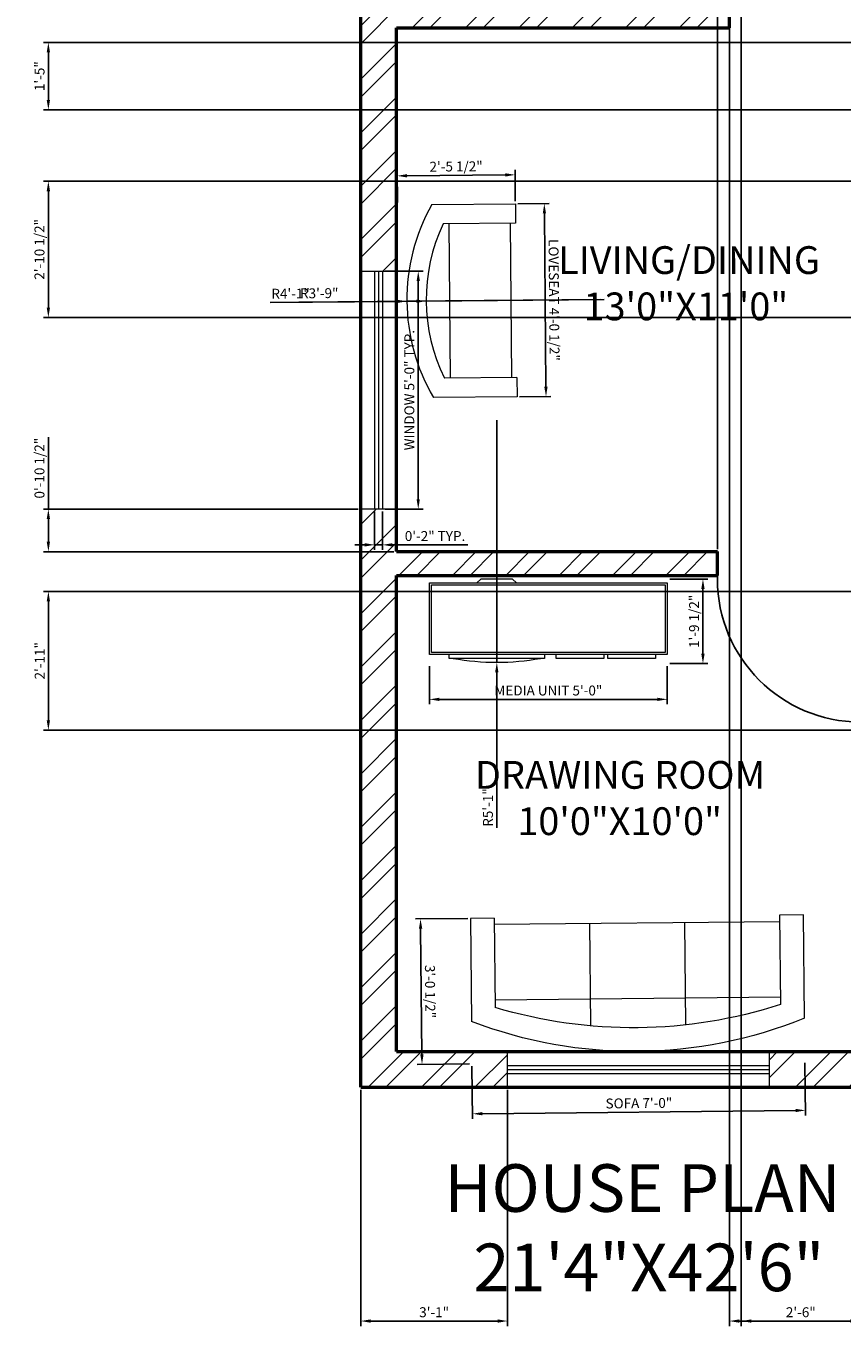
# Model space of a CAD drawing. Units: inches. Extents: x 1147 to 1568, y 1982 to 2559.
# Tile 1 of 4: x 1147 to 1353, y 1982 to 2309. Entities that reach past the tile are written whole.
import ezdxf

# ---------------------------------------------------------------- set-up
doc = ezdxf.new("R2010")
doc.units = ezdxf.units.IN
for name, color, linetype, lineweight in [('A-ANNO-DIMS', 2, 'Continuous', 18), ('A-DOOR', 4, 'Continuous', 25), ('A-WALL', 7, 'Continuous', 50), ('A-WALL-PATT', 252, 'Continuous', 13)]:
    doc.layers.add(name, color=color, linetype=linetype, lineweight=lineweight)
for name, color, linetype, lineweight, true_color in [('A-ANNO-TITL', 244, 'Continuous', 35, 0x991b1e), ('A-AREA-IDEN', 244, 'Continuous', 25, 0x991b1e), ('A-FURN', 244, 'Continuous', 18, 0x991b1e), ('A-GLAZ', 177, 'Continuous', 18, 0x293189)]:
    doc.layers.add(name, color=color, linetype=linetype, lineweight=lineweight, true_color=true_color)
doc.styles.get("Standard").update_dxf_attribs({"font": 'arial.ttf'})
doc.dimstyles.new('ISO-25', dxfattribs={"dimtxt": 2.5, "dimasz": 2.5, "dimexe": 1.25, "dimexo": 0.625, "dimtad": 1, "dimlunit": 3, "dimtxsty": 'Standard', "dimcen": 2.5, "dimadec": 0, "dimazin": 0, "dimtfac": 1, "dimtmove": 0, "dimatfit": 3, "dimfxl": 1, "dimarcsym": 0})

# ---------------------------------------------------------------- blocks, each defined once
blk = doc.blocks.new('*U3')
for p, q in [((-40, 0), (-40, 6)), ((0, 0), (0, 6))]:
    blk.add_line(p, q)
blk.add_lwpolyline([(0, 0), (0, -40), (-1.75, -40), (-1.75, 0)], close=True)
blk.add_arc((0, 0), 40, 180, 270)
blk = doc.blocks.new('Entertainment Center')
for p, q in [((-4, 0), (-5, -1)), ((4, 0), (-4, 0)), ((5, -1), (4, 0)), ((-17, -19), (-17, -1)), ((-17, -1), (43, -1)), ((-16.5, -18.5), (-16.5, -1.5)), ((-16.5, -1.5), (42.5, -1.5)), ((42.5, -1.5), (42.5, -18.5)), ((43, -1), (43, -19)), ((43, -19), (-17, -19)), ((42.5, -18.5), (-16.5, -18.5)), ((-12, -20), (-12, -19)), ((12, -19), (12, -20)), ((15, -20), (15, -19)), ((27, -19), (27, -20)), ((28, -20), (28, -19)), ((40, -19), (40, -20)), ((12, -20), (-12, -20)), ((27, -20), (15, -20)), ((40, -20), (28, -20))]:
    blk.add_line(p, q)
blk.add_arc((0, 40), 61, 259.6111, 280.3889)
blk = doc.blocks.new('Sofa - Roundback Loveseat 5 ft.')
for p, q in [((0, -32.44198), (0, -5.99998)), ((-24, -33.99998), (-24, -11.46958)), ((24.00004, -33.99998), (24.00004, -11.46958)), ((-23.9998, -13.38178), (23.99986, -13.38178)), ((-24, -32.44198), (24.00004, -32.44198))]:
    blk.add_line(p, q)
for points in [[(-24, -33.99998), (-30, -33.99998), (-30, -7.99998)], [(30.00004, -7.99998), (30.00004, -33.99998), (24.00004, -33.99998)]]:
    blk.add_lwpolyline(points)
for centre, radius, start, end in [((0, -60.24998), 60.24998, 60.13715, 119.8628), ((0, -61.38438), 55.38444, 64.32083, 115.6792)]:
    blk.add_arc(centre, radius, start, end)
blk = doc.blocks.new('Sofa - Roundback 7 ft.')
for p, q in [((-12.00002, -32.4421), (-12.00003, -6.5971)), ((11.99997, -32.4421), (11.99998, -6.5971)), ((-36.000027, -34), (-36.000027, -11.4696)), ((35.99998, -34), (35.99998, -11.4696)), ((-35.999844, -13.3819), (35.9998, -13.3819)), ((-36.000027, -32.4421), (35.99998, -32.4421))]:
    blk.add_line(p, q)
for points in [[(-36.000027, -34), (-42.000027, -34), (-42.000027, -8)], [(41.99998, -8), (41.99998, -34), (35.99998, -34)]]:
    blk.add_lwpolyline(points)
for centre, radius, start, end in [((0, -114.25), 114.25, 68.43141, 111.5686), ((-0.00001, -127.1968), 121.1968, 72.72033, 107.2797)]:
    blk.add_arc(centre, radius, start, end)
blk = doc.blocks.new('WIN-GLAZ-66IN')
for p, q in [((0, 2), (66, 2)), ((0, 1), (66, 1)), ((0, 0), (66, 0))]:
    blk.add_line(p, q)
blk = doc.blocks.new('WIN-GLAZ-60IN')
for p, q in [((0, 60), (0, 0)), ((1, 60), (1, 0)), ((2, 60), (2, 0))]:
    blk.add_line(p, q)
blk = doc.blocks.new('*D25')
at = {"layer": 'A-ANNO-DIMS', "color": 0, "lineweight": -2, "transparency": 16777216}
for p, q in [((1237.73, 2247.42), (1247.36, 2247.42)), ((1246.11, 2189.92), (1246.11, 2244.92)), ((1237.73, 2187.42), (1247.36, 2187.42))]:
    blk.add_line(p, q, dxfattribs=at)
at = {"layer": 'A-ANNO-DIMS', "color": 0, "transparency": 16777216}
for points in [[(1245.69, 2244.92), (1246.52, 2244.92), (1246.11, 2247.42)], [(1245.69, 2189.92), (1246.52, 2189.92), (1246.11, 2187.42)]]:
    blk.add_solid(points, dxfattribs=at)
at = {"layer": 'Defpoints', "color": 0, "transparency": 16777216}
for p in [(1237.11, 2247.42), (1246.11, 2247.42), (1237.11, 2187.42)]:
    blk.add_point(p, dxfattribs=at)
at = {"layer": 'A-ANNO-DIMS', "color": 0, "transparency": 16777216, "insert": (1244.19, 2217.42), "char_height": 2.5, "attachment_point": 5, "rotation": 90}
blk.add_mtext('WINDOW 5\'-0" TYP.', dxfattribs=at)
blk = doc.blocks.new('*D26')
at = {"layer": 'A-ANNO-DIMS', "color": 0, "lineweight": -2, "transparency": 16777216}
for p, q in [((1235.11, 2186.79), (1235.11, 2177.17)), ((1237.11, 2186.79), (1237.11, 2177.17)), ((1232.61, 2178.42), (1230.11, 2178.42)), ((1235.11, 2178.42), (1237.11, 2178.42)), ((1239.61, 2178.42), (1258.6, 2178.42))]:
    blk.add_line(p, q, dxfattribs=at)
at = {"layer": 'A-ANNO-DIMS', "color": 0, "transparency": 16777216}
for points in [[(1232.61, 2178.84), (1232.61, 2178), (1235.11, 2178.42)], [(1239.61, 2178.84), (1239.61, 2178), (1237.11, 2178.42)]]:
    blk.add_solid(points, dxfattribs=at)
at = {"layer": 'Defpoints', "color": 0, "transparency": 16777216}
for p in [(1235.11, 2187.42), (1237.11, 2187.42), (1237.11, 2178.42)]:
    blk.add_point(p, dxfattribs=at)
at = {"layer": 'A-ANNO-DIMS', "color": 0, "transparency": 16777216, "insert": (1250.35, 2180.32), "char_height": 2.5, "attachment_point": 5}
blk.add_mtext('0\'-2" TYP.', dxfattribs=at)
blk = doc.blocks.new('*D35')
at = {"layer": 'A-ANNO-DIMS', "color": 0, "lineweight": -2, "transparency": 16777216}
for p, q in [((1248.93, 2147.85), (1248.93, 2138.23)), ((1308.93, 2147.85), (1308.93, 2138.23)), ((1251.43, 2139.48), (1306.43, 2139.48))]:
    blk.add_line(p, q, dxfattribs=at)
at = {"layer": 'A-ANNO-DIMS', "color": 0, "transparency": 16777216}
for points in [[(1251.43, 2139.89), (1251.43, 2139.06), (1248.93, 2139.48)], [(1306.43, 2139.89), (1306.43, 2139.06), (1308.93, 2139.48)]]:
    blk.add_solid(points, dxfattribs=at)
at = {"layer": 'Defpoints', "color": 0, "transparency": 16777216}
for p in [(1248.93, 2148.48), (1308.93, 2148.48), (1308.93, 2139.48)]:
    blk.add_point(p, dxfattribs=at)
at = {"layer": 'A-ANNO-DIMS', "color": 0, "transparency": 16777216, "insert": (1278.93, 2141.38), "char_height": 2.5, "attachment_point": 5}
blk.add_mtext('MEDIA UNIT 5\'-0"', dxfattribs=at)
blk = doc.blocks.new('*D36')
at = {"layer": 'A-ANNO-DIMS', "color": 0, "lineweight": -2, "transparency": 16777216}
for p, q in [((1309.55, 2169.81), (1319.18, 2169.81)), ((1317.93, 2150.98), (1317.93, 2167.31)), ((1309.55, 2148.48), (1319.18, 2148.48))]:
    blk.add_line(p, q, dxfattribs=at)
at = {"layer": 'A-ANNO-DIMS', "color": 0, "transparency": 16777216}
for points in [[(1317.51, 2167.31), (1318.34, 2167.31), (1317.93, 2169.81)], [(1317.51, 2150.98), (1318.34, 2150.98), (1317.93, 2148.48)]]:
    blk.add_solid(points, dxfattribs=at)
at = {"layer": 'Defpoints', "color": 0, "transparency": 16777216}
for p in [(1308.93, 2169.81), (1317.93, 2169.81), (1308.93, 2148.48)]:
    blk.add_point(p, dxfattribs=at)
at = {"layer": 'A-ANNO-DIMS', "color": 0, "transparency": 16777216, "insert": (1316.01, 2159.14), "char_height": 2.5, "attachment_point": 5, "rotation": 90}
blk.add_mtext('1\'-9 1/2"', dxfattribs=at)
blk = doc.blocks.new('*D39')
at = {"layer": 'A-ANNO-DIMS', "color": 0, "lineweight": -2, "transparency": 16777216}
for p, q in [((1271.23, 2264.4), (1279.16, 2264.47)), ((1278.32, 2218.29), (1277.93, 2261.96)), ((1271.67, 2215.73), (1279.59, 2215.8))]:
    blk.add_line(p, q, dxfattribs=at)
at = {"layer": 'A-ANNO-DIMS', "color": 0, "transparency": 16777216}
for points in [[(1278.35, 2261.96), (1277.52, 2261.95), (1277.91, 2264.46)], [(1278.74, 2218.29), (1277.9, 2218.29), (1278.34, 2215.79)]]:
    blk.add_solid(points, dxfattribs=at)
at = {"layer": 'Defpoints', "color": 0, "transparency": 16777216}
for p in [(1270.61, 2264.39), (1277.91, 2264.46), (1271.04, 2215.72)]:
    blk.add_point(p, dxfattribs=at)
at = {"layer": 'A-ANNO-DIMS', "color": 0, "transparency": 16777216, "insert": (1280.04, 2240.14), "char_height": 2.5, "attachment_point": 5, "rotation": 270.5097}
blk.add_mtext('LOVESEAT 4\'-0 1/2"', dxfattribs=at)
blk = doc.blocks.new('*D40')
at = {"layer": 'A-ANNO-DIMS', "color": 0, "lineweight": -2, "transparency": 16777216}
for p, q in [((1240.86, 2264.75), (1240.79, 2272.68)), ((1268.05, 2271.67), (1243.3, 2271.45)), ((1270.6, 2265.02), (1270.53, 2272.94))]:
    blk.add_line(p, q, dxfattribs=at)
at = {"layer": 'A-ANNO-DIMS', "color": 0, "transparency": 16777216}
for points in [[(1243.3, 2271.87), (1243.31, 2271.03), (1240.8, 2271.43)], [(1268.04, 2272.09), (1268.05, 2271.25), (1270.54, 2271.69)]]:
    blk.add_solid(points, dxfattribs=at)
at = {"layer": 'Defpoints', "color": 0, "transparency": 16777216}
for p in [(1240.8, 2271.43), (1270.61, 2264.39), (1240.87, 2264.13)]:
    blk.add_point(p, dxfattribs=at)
at = {"layer": 'A-ANNO-DIMS', "color": 0, "transparency": 16777216, "insert": (1255.66, 2273.48), "char_height": 2.5, "attachment_point": 5, "rotation": 0.5097}
blk.add_mtext('2\'-5 1/2"', dxfattribs=at)
blk = doc.blocks.new('*D41')
at = {"layer": 'A-ANNO-DIMS', "color": 0, "lineweight": -2, "transparency": 16777216}
for p, q in [((1259.67, 2046.98), (1259.8, 2033.76)), ((1343.66, 2047.85), (1343.8, 2034.62)), ((1262.29, 2035.03), (1341.29, 2035.85))]:
    blk.add_line(p, q, dxfattribs=at)
at = {"layer": 'A-ANNO-DIMS', "color": 0, "transparency": 16777216}
for points in [[(1262.29, 2035.45), (1262.29, 2034.62), (1259.79, 2035.01)], [(1341.28, 2036.26), (1341.29, 2035.43), (1343.79, 2035.87)]]:
    blk.add_solid(points, dxfattribs=at)
at = {"layer": 'Defpoints', "color": 0, "transparency": 16777216}
for p in [(1343.66, 2048.47), (1259.66, 2047.61), (1343.79, 2035.87)]:
    blk.add_point(p, dxfattribs=at)
at = {"layer": 'A-ANNO-DIMS', "color": 0, "transparency": 16777216, "insert": (1301.77, 2037.36), "char_height": 2.5, "attachment_point": 5, "rotation": 0.59}
blk.add_mtext('SOFA 7\'-0"', dxfattribs=at)
blk = doc.blocks.new('*D42')
at = {"layer": 'A-ANNO-DIMS', "color": 0, "lineweight": -2, "transparency": 16777216}
for p, q in [((1258.66, 2084.26), (1245.43, 2084.13)), ((1246.71, 2081.64), (1247.03, 2049.98)), ((1259.03, 2047.6), (1245.81, 2047.46))]:
    blk.add_line(p, q, dxfattribs=at)
at = {"layer": 'A-ANNO-DIMS', "color": 0, "transparency": 16777216}
for points in [[(1247.13, 2081.64), (1246.29, 2081.64), (1246.68, 2084.14)], [(1247.45, 2049.98), (1246.62, 2049.97), (1247.06, 2047.48)]]:
    blk.add_solid(points, dxfattribs=at)
at = {"layer": 'Defpoints', "color": 0, "transparency": 16777216}
for p in [(1259.28, 2084.27), (1247.06, 2047.48), (1259.66, 2047.61)]:
    blk.add_point(p, dxfattribs=at)
at = {"layer": 'A-ANNO-DIMS', "color": 0, "transparency": 16777216, "insert": (1248.79, 2065.83), "char_height": 2.5, "attachment_point": 5, "rotation": 270.59}
blk.add_mtext('3\'-0 1/2"', dxfattribs=at)
blk = doc.blocks.new('*D43')
at = {"layer": 'A-ANNO-DIMS', "color": 0, "lineweight": -2, "transparency": 16777216}
for p, q in [((1327.61, 2368.08), (1327.61, 1981.52)), ((1357.61, 2368.08), (1357.61, 1981.52)), ((1330.11, 1982.77), (1355.11, 1982.77))]:
    blk.add_line(p, q, dxfattribs=at)
at = {"layer": 'A-ANNO-DIMS', "color": 0, "transparency": 16777216}
for points in [[(1330.11, 1983.19), (1330.11, 1982.35), (1327.61, 1982.77)], [(1355.11, 1983.19), (1355.11, 1982.35), (1357.61, 1982.77)]]:
    blk.add_solid(points, dxfattribs=at)
at = {"layer": 'Defpoints', "color": 0, "transparency": 16777216}
for p in [(1327.61, 2368.7), (1357.61, 2368.7), (1357.61, 1982.77)]:
    blk.add_point(p, dxfattribs=at)
at = {"layer": 'A-ANNO-DIMS', "color": 0, "transparency": 16777216, "insert": (1342.61, 1984.67), "char_height": 2.5, "attachment_point": 5}
blk.add_mtext('2\'-6"', dxfattribs=at)
blk = doc.blocks.new('*D45')
at = {"layer": 'A-ANNO-DIMS', "color": 0, "lineweight": -2, "transparency": 16777216}
for p, q in [((1321.61, 2177.33), (1321.61, 2556.75)), ((1357.61, 2177.33), (1357.61, 2556.75)), ((1324.11, 2555.5), (1355.11, 2555.5))]:
    blk.add_line(p, q, dxfattribs=at)
at = {"layer": 'A-ANNO-DIMS', "color": 0, "transparency": 16777216}
for points in [[(1324.11, 2555.92), (1324.11, 2555.09), (1321.61, 2555.5)], [(1355.11, 2555.92), (1355.11, 2555.09), (1357.61, 2555.5)]]:
    blk.add_solid(points, dxfattribs=at)
at = {"layer": 'Defpoints', "color": 0, "transparency": 16777216}
for p in [(1357.61, 2555.5), (1321.61, 2176.7), (1357.61, 2176.7)]:
    blk.add_point(p, dxfattribs=at)
at = {"layer": 'A-ANNO-DIMS', "color": 0, "transparency": 16777216, "insert": (1339.61, 2557.41), "char_height": 2.5, "attachment_point": 5}
blk.add_mtext('3\'-0"', dxfattribs=at)
blk = doc.blocks.new('*D48')
at = {"layer": 'A-ANNO-DIMS', "color": 0, "lineweight": -2, "transparency": 16777216}
for p, q in [((1391.98, 2166.7), (1151.56, 2166.7)), ((1152.81, 2134.2), (1152.81, 2164.2)), ((1391.98, 2131.7), (1151.56, 2131.7))]:
    blk.add_line(p, q, dxfattribs=at)
at = {"layer": 'A-ANNO-DIMS', "color": 0, "transparency": 16777216}
for points in [[(1152.39, 2164.2), (1153.22, 2164.2), (1152.81, 2166.7)], [(1152.39, 2134.2), (1153.22, 2134.2), (1152.81, 2131.7)]]:
    blk.add_solid(points, dxfattribs=at)
at = {"layer": 'Defpoints', "color": 0, "transparency": 16777216}
for p in [(1152.81, 2166.7), (1392.61, 2166.7), (1392.61, 2131.7)]:
    blk.add_point(p, dxfattribs=at)
at = {"layer": 'A-ANNO-DIMS', "color": 0, "transparency": 16777216, "insert": (1150.93, 2149.2), "char_height": 2.5, "attachment_point": 5, "rotation": 90}
blk.add_mtext('2\'-11"', dxfattribs=at)
blk = doc.blocks.new('*D55')
at = {"layer": 'A-ANNO-DIMS', "color": 0, "lineweight": -2, "transparency": 16777216}
for p, q in [((1231.61, 2041.08), (1231.61, 1981.52)), ((1268.63, 2041.08), (1268.63, 1981.52)), ((1234.11, 1982.77), (1266.13, 1982.77))]:
    blk.add_line(p, q, dxfattribs=at)
at = {"layer": 'A-ANNO-DIMS', "color": 0, "transparency": 16777216}
for points in [[(1234.11, 1983.19), (1234.11, 1982.35), (1231.61, 1982.77)], [(1266.13, 1983.19), (1266.13, 1982.35), (1268.63, 1982.77)]]:
    blk.add_solid(points, dxfattribs=at)
at = {"layer": 'Defpoints', "color": 0, "transparency": 16777216}
for p in [(1231.61, 2041.7), (1268.63, 2041.7), (1268.63, 1982.77)]:
    blk.add_point(p, dxfattribs=at)
at = {"layer": 'A-ANNO-DIMS', "color": 0, "transparency": 16777216, "insert": (1250.12, 1984.67), "char_height": 2.5, "attachment_point": 5}
blk.add_mtext('3\'-1"', dxfattribs=at)
blk = doc.blocks.new('*D57')
at = {"layer": 'A-ANNO-DIMS', "color": 0, "lineweight": -2, "transparency": 16777216}
for p, q in [((1152.81, 2187.42), (1152.81, 2205.58)), ((1230.98, 2187.42), (1151.56, 2187.42)), ((1152.81, 2179.2), (1152.81, 2184.92)), ((1239.98, 2176.7), (1151.56, 2176.7))]:
    blk.add_line(p, q, dxfattribs=at)
at = {"layer": 'A-ANNO-DIMS', "color": 0, "transparency": 16777216}
for points in [[(1152.39, 2184.92), (1153.22, 2184.92), (1152.81, 2187.42)], [(1152.39, 2179.2), (1153.22, 2179.2), (1152.81, 2176.7)]]:
    blk.add_solid(points, dxfattribs=at)
at = {"layer": 'Defpoints', "color": 0, "transparency": 16777216}
for p in [(1152.81, 2187.42), (1231.61, 2187.42), (1240.61, 2176.7)]:
    blk.add_point(p, dxfattribs=at)
at = {"layer": 'A-ANNO-DIMS', "color": 0, "transparency": 16777216, "insert": (1150.89, 2197.75), "char_height": 2.5, "attachment_point": 5, "rotation": 90}
blk.add_mtext('0\'-10 1/2"', dxfattribs=at)
blk = doc.blocks.new('*D62')
at = {"layer": 'A-ANNO-DIMS', "color": 0, "lineweight": -2, "transparency": 16777216}
for p, q in [((1324.61, 2335.08), (1324.61, 1981.52)), ((1400.61, 2335.08), (1400.61, 1981.52)), ((1327.11, 1982.77), (1398.11, 1982.77))]:
    blk.add_line(p, q, dxfattribs=at)
at = {"layer": 'A-ANNO-DIMS', "color": 0, "transparency": 16777216}
for points in [[(1327.11, 1983.19), (1327.11, 1982.35), (1324.61, 1982.77)], [(1398.11, 1983.19), (1398.11, 1982.35), (1400.61, 1982.77)]]:
    blk.add_solid(points, dxfattribs=at)
at = {"layer": 'Defpoints', "color": 0, "transparency": 16777216}
for p in [(1324.61, 2335.7), (1400.61, 2335.7), (1400.61, 1982.77)]:
    blk.add_point(p, dxfattribs=at)
at = {"layer": 'A-ANNO-DIMS', "color": 0, "transparency": 16777216, "insert": (1362.61, 1984.67), "char_height": 2.5, "attachment_point": 5}
blk.add_mtext('6\'-4"', dxfattribs=at)
blk = doc.blocks.new('*D66')
at = {"layer": 'A-ANNO-DIMS', "color": 0, "lineweight": -2, "transparency": 16777216}
for p, q in [((1458.15, 2270.07), (1151.56, 2270.07)), ((1152.81, 2238.23), (1152.81, 2267.57)), ((1458.15, 2235.73), (1151.56, 2235.73))]:
    blk.add_line(p, q, dxfattribs=at)
at = {"layer": 'A-ANNO-DIMS', "color": 0, "transparency": 16777216}
for points in [[(1152.39, 2267.57), (1153.22, 2267.57), (1152.81, 2270.07)], [(1152.39, 2238.23), (1153.22, 2238.23), (1152.81, 2235.73)]]:
    blk.add_solid(points, dxfattribs=at)
at = {"layer": 'Defpoints', "color": 0, "transparency": 16777216}
for p in [(1152.81, 2270.07), (1458.78, 2270.07), (1458.78, 2235.73)]:
    blk.add_point(p, dxfattribs=at)
at = {"layer": 'A-ANNO-DIMS', "color": 0, "transparency": 16777216, "insert": (1150.89, 2252.9), "char_height": 2.5, "attachment_point": 5, "rotation": 90}
blk.add_mtext('2\'-10 1/2"', dxfattribs=at)
blk = doc.blocks.new('*D68')
at = {"layer": 'A-ANNO-DIMS', "color": 0, "lineweight": -2, "transparency": 16777216}
for p, q in [((1416.1, 2305.06), (1151.56, 2305.06)), ((1152.81, 2302.56), (1152.81, 2290.56)), ((1416.1, 2288.06), (1151.56, 2288.06))]:
    blk.add_line(p, q, dxfattribs=at)
at = {"layer": 'A-ANNO-DIMS', "color": 0, "transparency": 16777216}
for points in [[(1152.39, 2302.56), (1153.22, 2302.56), (1152.81, 2305.06)], [(1152.39, 2290.56), (1153.22, 2290.56), (1152.81, 2288.06)]]:
    blk.add_solid(points, dxfattribs=at)
at = {"layer": 'Defpoints', "color": 0, "transparency": 16777216}
for p in [(1416.72, 2305.06), (1152.81, 2288.06), (1416.72, 2288.06)]:
    blk.add_point(p, dxfattribs=at)
at = {"layer": 'A-ANNO-DIMS', "color": 0, "transparency": 16777216, "insert": (1150.91, 2296.56), "char_height": 2.5, "attachment_point": 5, "rotation": 90}
blk.add_mtext('1\'-5"', dxfattribs=at)
blk = doc.blocks.new('*D69')
at = {"layer": 'A-ANNO-DIMS', "color": 0, "lineweight": -2, "transparency": 16777216}
for p, q in [((1265.93, 2209.81), (1265.93, 2148.81)), ((1265.93, 2107.07), (1265.93, 2146.31))]:
    blk.add_line(p, q, dxfattribs=at)
at = {"layer": 'A-ANNO-DIMS', "color": 0, "transparency": 16777216}
blk.add_solid([(1265.51, 2146.31), (1266.34, 2146.31), (1265.93, 2148.81)], dxfattribs=at)
at = {"layer": 'Defpoints', "color": 0, "transparency": 16777216}
for p in [(1265.93, 2209.81), (1265.93, 2148.81)]:
    blk.add_point(p, dxfattribs=at)
at = {"layer": 'A-ANNO-DIMS', "color": 0, "transparency": 16777216, "insert": (1264.02, 2112.21), "char_height": 2.5, "attachment_point": 5, "rotation": 89.9998}
blk.add_mtext('R5\'-1"', dxfattribs=at)
blk = doc.blocks.new('*D70')
at = {"layer": 'A-ANNO-DIMS', "color": 0, "lineweight": -2, "transparency": 16777216}
for p, q in [((1208.78, 2239.51), (1240.75, 2239.79)), ((1292.12, 2240.25), (1243.25, 2239.81))]:
    blk.add_line(p, q, dxfattribs=at)
at = {"layer": 'A-ANNO-DIMS', "color": 0, "transparency": 16777216}
blk.add_solid([(1240.74, 2240.21), (1240.75, 2239.37), (1243.25, 2239.81)], dxfattribs=at)
at = {"layer": 'Defpoints', "color": 0, "transparency": 16777216}
for p in [(1243.25, 2239.81), (1292.12, 2240.25)]:
    blk.add_point(p, dxfattribs=at)
at = {"layer": 'A-ANNO-DIMS', "color": 0, "transparency": 16777216, "insert": (1213.91, 2241.43), "char_height": 2.5, "attachment_point": 5, "rotation": 0.5103}
blk.add_mtext('R4\'-1"', dxfattribs=at)
blk = doc.blocks.new('*D71')
at = {"layer": 'A-ANNO-DIMS', "color": 0, "lineweight": -2, "transparency": 16777216}
for p, q in [((1216.02, 2239.57), (1245.61, 2239.83)), ((1293.04, 2240.26), (1248.11, 2239.86))]:
    blk.add_line(p, q, dxfattribs=at)
at = {"layer": 'A-ANNO-DIMS', "color": 0, "transparency": 16777216}
blk.add_solid([(1245.61, 2240.25), (1245.62, 2239.42), (1248.11, 2239.86)], dxfattribs=at)
at = {"layer": 'Defpoints', "color": 0, "transparency": 16777216}
for p in [(1248.11, 2239.86), (1293.04, 2240.26)]:
    blk.add_point(p, dxfattribs=at)
at = {"layer": 'A-ANNO-DIMS', "color": 0, "transparency": 16777216, "insert": (1221.14, 2241.52), "char_height": 2.5, "attachment_point": 5, "rotation": 0.5094}
blk.add_mtext('R3\'-9"', dxfattribs=at)

msp = doc.modelspace()

# ---------------------------------------------------------------- hatches: boundary and pattern name
at = {"layer": 'A-WALL-PATT'}
h = msp.add_hatch(dxfattribs=at)
h.set_pattern_fill('ANSI32', color=256)
h.paths.add_polyline_path([(1240.607, 2518.704), (1268.63, 2518.704), (1268.63, 2527.704), (1231.607, 2527.704), (1231.607, 2348.295), (1240.607, 2348.295), (1240.607, 2368.704), (1318.607, 2368.704), (1318.607, 2365.704), (1324.607, 2365.704), (1324.607, 2368.704), (1327.607, 2368.704), (1327.607, 2374.704), (1240.607, 2374.704)])
h.paths.add_polyline_path([(1324.607, 2335.704), (1318.607, 2335.704), (1318.607, 2314.704), (1240.607, 2314.704), (1240.607, 2324.295), (1231.607, 2324.295), (1231.607, 2247.419), (1240.607, 2247.419), (1240.607, 2308.704), (1324.607, 2308.704)])
h.paths.add_polyline_path([(1487.607, 2527.704), (1464.679, 2527.704), (1464.679, 2518.704), (1478.607, 2518.704), (1478.607, 2374.704), (1399.607, 2374.704), (1399.607, 2368.704), (1400.607, 2368.704), (1400.607, 2365.704), (1406.607, 2365.704), (1406.607, 2368.704), (1478.607, 2368.704), (1478.607, 2343.549), (1487.607, 2343.549)])
h.paths.add_polyline_path([(1366.607, 2518.704), (1398.679, 2518.704), (1398.679, 2527.704), (1334.63, 2527.704), (1334.63, 2518.704), (1360.607, 2518.704), (1360.607, 2374.704), (1357.607, 2374.704), (1357.607, 2368.704), (1369.607, 2368.704), (1369.607, 2374.704), (1366.607, 2374.704)])
h.paths.add_polyline_path([(1487.607, 2319.549), (1478.607, 2319.549), (1478.607, 2314.704), (1406.607, 2314.704), (1406.607, 2335.704), (1400.607, 2335.704), (1400.607, 2308.704), (1406.607, 2308.704), (1406.607, 2284.704), (1412.607, 2284.704), (1412.607, 2308.704), (1478.607, 2308.704), (1478.607, 2295.917), (1487.607, 2295.917)])
h.paths.add_polyline_path([(1487.607, 2235.917), (1478.607, 2235.917), (1478.607, 2212.704), (1400.607, 2212.704), (1400.607, 2206.704), (1478.607, 2206.704), (1478.607, 2131.704), (1405.607, 2131.704), (1405.607, 2122.704), (1487.607, 2122.704)])
h.paths.add_polyline_path([(1369.607, 2122.704), (1369.607, 2131.704), (1366.607, 2131.704), (1366.607, 2176.704), (1357.607, 2176.704), (1357.607, 2170.704), (1360.607, 2170.704), (1360.607, 2050.704), (1334.63, 2050.704), (1334.63, 2041.704), (1369.607, 2041.704)])
h.paths.add_polyline_path([(1240.607, 2170.704), (1321.607, 2170.704), (1321.607, 2176.704), (1240.607, 2176.704), (1240.607, 2187.419), (1231.607, 2187.419), (1231.607, 2041.704), (1268.63, 2041.704), (1268.63, 2050.704), (1240.607, 2050.704)])

# ---------------------------------------------------------------- linework, layer by layer
at = {"layer": 'A-GLAZ'}
for points in [[(1231.607, 2247.419), (1240.607, 2247.419), (1240.607, 2187.419), (1231.607, 2187.419)], [(1268.63, 2050.704), (1334.63, 2050.704), (1334.63, 2041.704), (1268.63, 2041.704)]]:
    msp.add_lwpolyline(points, close=True, dxfattribs=at)
at = {"layer": 'A-WALL'}
for p, q in [((1231.607, 2041.704), (1231.607, 2527.704)), ((1324.607, 2308.704), (1324.607, 2335.704)), ((1240.607, 2308.704), (1324.607, 2308.704)), ((1240.607, 2176.704), (1240.607, 2308.704)), ((1240.607, 2176.704), (1321.607, 2176.704)), ((1321.607, 2170.704), (1321.607, 2176.704)), ((1240.607, 2050.704), (1240.607, 2170.704)), ((1240.607, 2170.704), (1321.607, 2170.704)), ((1240.607, 2050.704), (1360.607, 2050.704)), ((1231.607, 2041.704), (1369.607, 2041.704))]:
    msp.add_line(p, q, dxfattribs=at)

# ---------------------------------------------------------------- block references
at = {"layer": 'A-DOOR', "xscale": 0.9007809112098129, "yscale": 0.9007809112098129, "zscale": 0.9007809112098129}
msp.add_blockref('*U3', (1357.607, 2169.8), dxfattribs=at)
at = {"layer": 'A-FURN', "xscale": 0.8111609601354917, "yscale": 0.8111609601354917, "zscale": 0.8111609601354917, "rotation": 90.50972243052306}
msp.add_blockref('Sofa - Roundback Loveseat 5 ft.', (1243.248, 2239.812), dxfattribs=at)
at = {"layer": 'A-FURN'}
msp.add_blockref('Entertainment Center', (1265.926, 2169.81), dxfattribs=at)
at = {"layer": 'A-FURN', "xscale": -1, "rotation": 180.5899561012461}
msp.add_blockref('Sofa - Roundback 7 ft.', (1301.63, 2050.704), dxfattribs=at)
at = {"layer": 'A-GLAZ'}
for name, p in [('WIN-GLAZ-60IN', (1235.107, 2187.419)), ('WIN-GLAZ-66IN', (1268.63, 2045.204))]:
    msp.add_blockref(name, p, dxfattribs=at)

# ---------------------------------------------------------------- texts
at = {"layer": 'A-ANNO-TITL', "insert": (1249.023, 2022.295), "char_height": 12, "attachment_point": 1}
msp.add_mtext_dynamic_manual_height_columns('{ HOUSE PLAN\\P   21\'4"X42\'6"}', width=115.97351, gutter_width=12.5, heights=[0], dxfattribs=at)
at = {"layer": 'A-AREA-IDEN', "char_height": 7, "attachment_point": 1}
for s, width, insert in [('{LIVING/DINING\\P   13\'0"X11\'0"}', 68.59921, (1281.396, 2253.697)), ('{DRAWING ROOM\\P     10\'0"X10\'0"}', 79.10552, (1260.402, 2123.939))]:
    msp.add_mtext_dynamic_manual_height_columns(s, width=width, gutter_width=12.5, heights=[0], dxfattribs=dict(at, insert=insert))

# ---------------------------------------------------------------- dimensions: what is measured, and where the dimension line sits
at = {"layer": 'A-ANNO-DIMS'}
for base, p1, p2, picture, middle in [((1357.607, 2555.504), (1321.607, 2176.704), (1357.607, 2176.704), '*D45', (1339.607, 2557.407)), ((1357.607, 1982.772), (1327.607, 2368.704), (1357.607, 2368.704), '*D43', (1342.607, 1984.673)), ((1400.607, 1982.772), (1324.607, 2335.704), (1400.607, 2335.704), '*D62', (1362.607, 1984.673)), ((1268.63, 1982.772), (1231.607, 2041.704), (1268.63, 2041.704), '*D55', (1250.118, 1984.674))]:
    dim = msp.add_linear_dim(base=base, p1=p1, p2=p2, dimstyle='ISO-25', override={"dimdec": 1, "dimlfac": 1, "dimrnd": 0, "dimzin": 1, "dimdsep": 46, "dimlunit": 4, "dimfrac": 2}, dxfattribs=at)
    dim.commit()
    dim.dimension.update_dxf_attribs({"geometry": picture, "text_midpoint": middle})
for base, p1, p2, angle, picture, middle in [((1152.807, 2288.061), (1416.721, 2305.058), (1416.721, 2288.061), 90, '*D68', (1150.905, 2296.56)), ((1240.804, 2271.427), (1270.61, 2264.392), (1240.869, 2264.127), 180.50972, '*D40', (1255.657, 2273.477)), ((1152.807, 2270.074), (1458.779, 2235.728), (1458.779, 2270.074), 90, '*D66', (1150.889, 2252.901)), ((1152.807, 2187.419), (1240.607, 2176.704), (1231.607, 2187.419), 90, '*D57', (1150.889, 2197.751)), ((1317.926, 2169.81), (1308.926, 2148.476), (1308.926, 2169.81), 90, '*D36', (1316.009, 2159.143)), ((1152.807, 2166.704), (1392.607, 2131.704), (1392.607, 2166.704), 90, '*D48', (1150.927, 2149.204)), ((1247.06, 2047.476), (1259.282, 2084.27), (1259.66, 2047.605), 270.58996, '*D42', (1248.79, 2065.828))]:
    dim = msp.add_linear_dim(base=base, p1=p1, p2=p2, angle=angle, dimstyle='ISO-25', override={"dimdec": 1, "dimlfac": 1, "dimrnd": 0, "dimzin": 1, "dimdsep": 46, "dimlunit": 4, "dimfrac": 2}, dxfattribs=at)
    dim.commit()
    dim.dimension.update_dxf_attribs({"geometry": picture, "text_midpoint": middle})
for base, p1, p2, angle, text, picture, middle in [((1277.91, 2264.457), (1271.043, 2215.724), (1270.61, 2264.392), 90.50972, 'LOVESEAT <>', '*D39', (1280.045, 2240.14)), ((1246.107, 2247.419), (1237.107, 2187.419), (1237.107, 2247.419), 90, 'WINDOW <> TYP.', '*D25', (1244.188, 2217.419)), ((1343.785, 2035.871), (1259.66, 2047.605), (1343.655, 2048.47), 0.58996, 'SOFA <>', '*D41', (1301.768, 2037.357))]:
    dim = msp.add_linear_dim(base=base, p1=p1, p2=p2, angle=angle, text=text, dimstyle='ISO-25', override={"dimdec": 1, "dimlfac": 1, "dimrnd": 0, "dimzin": 1, "dimdsep": 46, "dimlunit": 4, "dimfrac": 2}, dxfattribs=at)
    dim.commit()
    dim.dimension.update_dxf_attribs({"geometry": picture, "text_midpoint": middle})
for center, mpoint, picture, middle in [((1292.119, 2240.247), (1243.248, 2239.812), '*D70', (1213.926, 2239.551)), ((1293.039, 2240.255), (1248.115, 2239.856), '*D71', (1221.16, 2239.616)), ((1265.926, 2209.81), (1265.926, 2148.81), '*D69', (1265.926, 2112.21))]:
    dim = msp.add_radius_dim(center=center, mpoint=mpoint, dimstyle='ISO-25', override={"dimdec": 1, "dimlfac": 1, "dimrnd": 0, "dimzin": 1, "dimdsep": 46, "dimlunit": 4, "dimfrac": 2}, dxfattribs=at)
    dim.commit()
    dim.dimension.update_dxf_attribs({"geometry": picture, "text_midpoint": middle, "dimtype": 164})
for base, p1, p2, text, picture, middle in [((1237.107, 2178.419), (1235.107, 2187.419), (1237.107, 2187.419), '<> TYP.', '*D26', (1250.351, 2180.321)), ((1308.926, 2139.476), (1248.926, 2148.476), (1308.926, 2148.476), 'MEDIA UNIT <>', '*D35', (1278.926, 2141.378))]:
    dim = msp.add_linear_dim(base=base, p1=p1, p2=p2, text=text, dimstyle='ISO-25', override={"dimdec": 1, "dimlfac": 1, "dimrnd": 0, "dimzin": 1, "dimdsep": 46, "dimlunit": 4, "dimfrac": 2}, dxfattribs=at)
    dim.commit()
    dim.dimension.update_dxf_attribs({"geometry": picture, "text_midpoint": middle})

doc.saveas('drawing.dxf')
